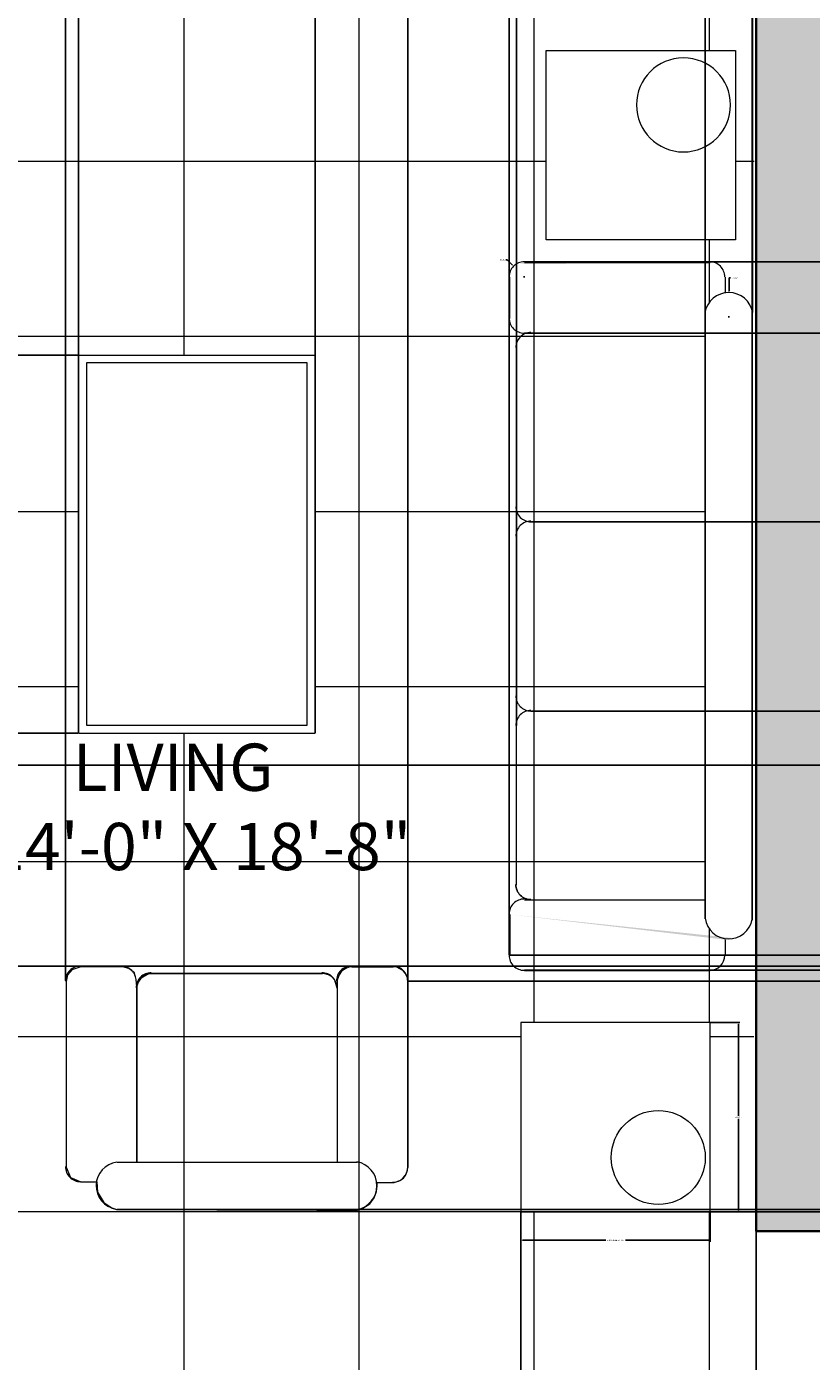
# Model space of a CAD drawing. Units: inches. Extents: x 6 to 575, y 34 to 566.
# Tile 15 of 21: x 282 to 382, y 262 to 432. Entities that reach past the tile are written whole.
import ezdxf

# ---------------------------------------------------------------- set-up
doc = ezdxf.new("R2010")
doc.units = ezdxf.units.IN
doc.linetypes.add('ACAD_ISO02W100', pattern=[15, 12, -3])
for name, color, linetype, lineweight in [('A-ANNO-DIMS', 2, 'Continuous', 18), ('A-AREA-IDEN', 6, 'Continuous', 20), ('A-FLOR-PATT', 252, 'Continuous', 9), ('A-WALL-OVHD', 7, 'ACAD_ISO02W100', 18), ('A-WALL-PATT', 251, 'Continuous', 9), ('FUR', 2, 'Continuous', 18), ('WALLS', 7, 'Continuous', 35)]:
    doc.layers.add(name, color=color, linetype=linetype, lineweight=lineweight)
doc.styles.add('PDF Arial Narrow', font='txt')
doc.styles.get("Standard").update_dxf_attribs({"font": 'arial.ttf'})
doc.dimstyles.get("Standard").update_dxf_attribs({"dimtxt": 0.18, "dimasz": 0.18, "dimexe": 0.18, "dimexo": 0.0625, "dimgap": 0.09, "dimtad": 0, "dimtih": 1, "dimtoh": 1, "dimdec": 4, "dimzin": 0, "dimdsep": 46, "dimtxsty": 'Standard', "dimcen": 0.09, "dimadec": 0, "dimazin": 0, "dimtfac": 1, "dimtdec": 4, "dimtofl": 0, "dimtmove": 0, "dimatfit": 3, "dimfxl": 1, "dimtolj": 1, "dimtzin": 0, "dimarcsym": 0})

# ---------------------------------------------------------------- blocks, each defined once
blk = doc.blocks.new('TABLE-END-24IN')
blk.add_lwpolyline([(24.03, 24.03), (0, 24.03), (0, 0), (24.03, 0)], close=True)
blk.add_circle((17.44, 6.9), 5.97)
blk = doc.blocks.new('*D27')
at = {"layer": 'A-ANNO-DIMS', "color": 0, "lineweight": -2, "transparency": 16777216}
for p, q in [((344.78, 281.17), (344.78, 277.45)), ((368.81, 281.17), (368.81, 277.45)), ((344.96, 277.63), (355.54, 277.63)), ((368.63, 277.63), (358.05, 277.63))]:
    blk.add_line(p, q, dxfattribs=at)
at = {"layer": 'A-ANNO-DIMS', "color": 0, "transparency": 16777216}
for points in [[(344.96, 277.66), (344.96, 277.6), (344.78, 277.63)], [(368.63, 277.66), (368.63, 277.6), (368.81, 277.63)]]:
    blk.add_solid(points, dxfattribs=at)
at = {"layer": 'Defpoints', "color": 0, "transparency": 16777216}
for p in [(344.78, 281.24), (368.81, 281.24), (368.81, 277.63)]:
    blk.add_point(p, dxfattribs=at)
at = {"layer": 'A-ANNO-DIMS', "color": 0, "transparency": 16777216, "insert": (356.79, 277.63), "char_height": 0.18, "attachment_point": 5}
blk.add_mtext('\\A1;END TABLE 24 TYP.', dxfattribs=at)
blk = doc.blocks.new('*D28')
at = {"layer": 'A-ANNO-DIMS', "color": 0, "lineweight": -2, "transparency": 16777216}
for p, q in [((368.87, 305.27), (372.59, 305.27)), ((372.41, 305.09), (372.41, 293.43)), ((372.41, 281.42), (372.41, 293.07)), ((368.87, 281.24), (372.59, 281.24))]:
    blk.add_line(p, q, dxfattribs=at)
at = {"layer": 'A-ANNO-DIMS', "color": 0, "transparency": 16777216}
for points in [[(372.38, 305.09), (372.44, 305.09), (372.41, 305.27)], [(372.38, 281.42), (372.44, 281.42), (372.41, 281.24)]]:
    blk.add_solid(points, dxfattribs=at)
at = {"layer": 'Defpoints', "color": 0, "transparency": 16777216}
for p in [(368.81, 305.27), (372.41, 305.27), (368.81, 281.24)]:
    blk.add_point(p, dxfattribs=at)
at = {"layer": 'A-ANNO-DIMS', "color": 0, "transparency": 16777216, "insert": (372.41, 293.25), "char_height": 0.18, "attachment_point": 5}
blk.add_mtext('\\A1;24 TYP.', dxfattribs=at)
blk = doc.blocks.new('*D54')
at = {"layer": 'A-ANNO-DIMS', "color": 0, "lineweight": -2, "transparency": 16777216}
for p, q in [((444.96, 337.94), (6.65, 337.94)), ((6.83, 337.76), (6.83, 299.11)), ((6.83, 260.1), (6.83, 298.75)), ((444.96, 259.92), (6.65, 259.92))]:
    blk.add_line(p, q, dxfattribs=at)
at = {"layer": 'A-ANNO-DIMS', "color": 0, "transparency": 16777216}
for points in [[(6.8, 337.76), (6.86, 337.76), (6.83, 337.94)], [(6.8, 260.1), (6.86, 260.1), (6.83, 259.92)]]:
    blk.add_solid(points, dxfattribs=at)
at = {"layer": 'Defpoints', "color": 0, "transparency": 16777216}
for p in [(6.83, 337.94), (445.02, 337.94), (445.02, 259.92)]:
    blk.add_point(p, dxfattribs=at)
at = {"layer": 'A-ANNO-DIMS', "color": 0, "transparency": 16777216, "insert": (6.83, 298.93), "char_height": 0.18, "attachment_point": 5}
blk.add_mtext('\\A1;78.02', dxfattribs=at)
blk = doc.blocks.new('*D119')
at = {"layer": 'A-ANNO-DIMS', "color": 0, "lineweight": -2, "transparency": 16777216}
for p, q in [((343.28, 400.02), (343.28, 565.81)), ((343.46, 565.63), (358.36, 565.63)), ((374.01, 565.63), (359.11, 565.63)), ((374.19, 395.44), (374.19, 565.81))]:
    blk.add_line(p, q, dxfattribs=at)
at = {"layer": 'A-ANNO-DIMS', "color": 0, "transparency": 16777216}
for points in [[(343.46, 565.66), (343.46, 565.6), (343.28, 565.63)], [(374.01, 565.66), (374.01, 565.6), (374.19, 565.63)]]:
    blk.add_solid(points, dxfattribs=at)
at = {"layer": 'Defpoints', "color": 0, "transparency": 16777216}
for p in [(374.19, 565.63), (343.28, 399.96), (374.19, 395.38)]:
    blk.add_point(p, dxfattribs=at)
at = {"layer": 'A-ANNO-DIMS', "color": 0, "transparency": 16777216, "insert": (358.73, 565.63), "char_height": 0.18, "attachment_point": 5}
blk.add_mtext('\\A1;30.91', dxfattribs=at)
blk = doc.blocks.new('*D120')
at = {"layer": 'A-ANNO-DIMS', "color": 0, "lineweight": -2, "transparency": 16777216}
for p, q in [((345.25, 401.87), (574.68, 401.87)), ((574.5, 401.69), (574.5, 357.07)), ((574.5, 312.09), (574.5, 356.71)), ((345.25, 311.91), (574.68, 311.91))]:
    blk.add_line(p, q, dxfattribs=at)
at = {"layer": 'A-ANNO-DIMS', "color": 0, "transparency": 16777216}
for points in [[(574.47, 401.69), (574.53, 401.69), (574.5, 401.87)], [(574.47, 312.09), (574.53, 312.09), (574.5, 311.91)]]:
    blk.add_solid(points, dxfattribs=at)
at = {"layer": 'Defpoints', "color": 0, "transparency": 16777216}
for p in [(345.19, 401.87), (574.5, 401.87), (345.19, 311.91)]:
    blk.add_point(p, dxfattribs=at)
at = {"layer": 'A-ANNO-DIMS', "color": 0, "transparency": 16777216, "insert": (574.5, 356.89), "char_height": 0.18, "attachment_point": 5}
blk.add_mtext('\\A1;89.96', dxfattribs=at)
blk = doc.blocks.new('*D121')
at = {"layer": 'A-ANNO-DIMS', "color": 0, "lineweight": -2, "transparency": 16777216}
for p, q in [((345.25, 311.91), (574.68, 311.91)), ((574.5, 311.73), (574.5, 296.75)), ((574.5, 281.42), (574.5, 296.39)), ((344.84, 281.24), (574.68, 281.24))]:
    blk.add_line(p, q, dxfattribs=at)
at = {"layer": 'A-ANNO-DIMS', "color": 0, "transparency": 16777216}
for points in [[(574.47, 311.73), (574.53, 311.73), (574.5, 311.91)], [(574.47, 281.42), (574.53, 281.42), (574.5, 281.24)]]:
    blk.add_solid(points, dxfattribs=at)
at = {"layer": 'Defpoints', "color": 0, "transparency": 16777216}
for p in [(345.19, 311.91), (574.5, 311.91), (344.78, 281.24)]:
    blk.add_point(p, dxfattribs=at)
at = {"layer": 'A-ANNO-DIMS', "color": 0, "transparency": 16777216, "insert": (574.5, 296.57), "char_height": 0.18, "attachment_point": 5}
blk.add_mtext('\\A1;30.673', dxfattribs=at)
blk = doc.blocks.new('*D122')
at = {"layer": 'A-ANNO-DIMS', "color": 0, "lineweight": -2, "transparency": 16777216}
for p, q in [((344.78, 281.17), (344.78, 33.76)), ((374.66, 278.74), (374.66, 33.76)), ((344.96, 33.94), (359.32, 33.94)), ((374.48, 33.94), (360.11, 33.94))]:
    blk.add_line(p, q, dxfattribs=at)
at = {"layer": 'A-ANNO-DIMS', "color": 0, "transparency": 16777216}
for points in [[(344.96, 33.97), (344.96, 33.91), (344.78, 33.94)], [(374.48, 33.97), (374.48, 33.91), (374.66, 33.94)]]:
    blk.add_solid(points, dxfattribs=at)
at = {"layer": 'Defpoints', "color": 0, "transparency": 16777216}
for p in [(344.78, 281.24), (374.66, 278.8), (344.78, 33.94)]:
    blk.add_point(p, dxfattribs=at)
at = {"layer": 'A-ANNO-DIMS', "color": 0, "transparency": 16777216, "insert": (359.72, 33.94), "char_height": 0.18, "attachment_point": 5}
blk.add_mtext('\\A1;29.88', dxfattribs=at)
blk = doc.blocks.new('*D123')
at = {"layer": 'A-ANNO-DIMS', "color": 0, "lineweight": -2, "transparency": 16777216}
for p, q in [((344.84, 281.24), (574.68, 281.24)), ((574.5, 281.06), (574.5, 280.2)), ((574.5, 278.98), (574.5, 279.84)), ((374.72, 278.8), (574.68, 278.8))]:
    blk.add_line(p, q, dxfattribs=at)
at = {"layer": 'A-ANNO-DIMS', "color": 0, "transparency": 16777216}
for points in [[(574.47, 281.06), (574.53, 281.06), (574.5, 281.24)], [(574.47, 278.98), (574.53, 278.98), (574.5, 278.8)]]:
    blk.add_solid(points, dxfattribs=at)
at = {"layer": 'Defpoints', "color": 0, "transparency": 16777216}
for p in [(344.78, 281.24), (574.5, 281.24), (374.66, 278.8)]:
    blk.add_point(p, dxfattribs=at)
at = {"layer": 'A-ANNO-DIMS', "color": 0, "transparency": 16777216, "insert": (574.5, 280.02), "char_height": 0.18, "attachment_point": 5}
blk.add_mtext('\\A1;2.435', dxfattribs=at)
blk = doc.blocks.new('*D124')
at = {"layer": 'A-ANNO-DIMS', "color": 0, "lineweight": -2, "transparency": 16777216}
for p, q in [((345.25, 401.87), (574.68, 401.87)), ((574.5, 401.69), (574.5, 397.53)), ((574.5, 393), (574.5, 397.16)), ((345.25, 392.82), (574.68, 392.82))]:
    blk.add_line(p, q, dxfattribs=at)
at = {"layer": 'A-ANNO-DIMS', "color": 0, "transparency": 16777216}
for points in [[(574.47, 401.69), (574.53, 401.69), (574.5, 401.87)], [(574.47, 393), (574.53, 393), (574.5, 392.82)]]:
    blk.add_solid(points, dxfattribs=at)
at = {"layer": 'Defpoints', "color": 0, "transparency": 16777216}
for p in [(345.19, 401.87), (574.5, 401.87), (345.19, 392.82)]:
    blk.add_point(p, dxfattribs=at)
at = {"layer": 'A-ANNO-DIMS', "color": 0, "transparency": 16777216, "insert": (574.5, 397.34), "char_height": 0.18, "attachment_point": 5}
blk.add_mtext('\\A1;9.05', dxfattribs=at)
blk = doc.blocks.new('*D125')
at = {"layer": 'A-ANNO-DIMS', "color": 0, "lineweight": -2, "transparency": 16777216}
for p, q in [((346.11, 368.87), (574.68, 368.87)), ((574.5, 368.69), (574.5, 357.03)), ((574.5, 345.01), (574.5, 356.67)), ((346.11, 344.83), (574.68, 344.83))]:
    blk.add_line(p, q, dxfattribs=at)
at = {"layer": 'A-ANNO-DIMS', "color": 0, "transparency": 16777216}
for points in [[(574.47, 368.69), (574.53, 368.69), (574.5, 368.87)], [(574.47, 345.01), (574.53, 345.01), (574.5, 344.83)]]:
    blk.add_solid(points, dxfattribs=at)
at = {"layer": 'Defpoints', "color": 0, "transparency": 16777216}
for p in [(346.05, 368.87), (574.5, 368.87), (346.05, 344.83)]:
    blk.add_point(p, dxfattribs=at)
at = {"layer": 'A-ANNO-DIMS', "color": 0, "transparency": 16777216, "insert": (574.5, 356.85), "char_height": 0.18, "attachment_point": 5}
blk.add_mtext('\\A1;24.03', dxfattribs=at)
blk = doc.blocks.new('*D126')
at = {"layer": 'A-ANNO-DIMS', "color": 0, "lineweight": -2, "transparency": 16777216}
for p, q in [((368.18, 318.51), (368.18, 565.81)), ((368.36, 565.63), (370.78, 565.63)), ((373.95, 565.63), (371.53, 565.63)), ((374.13, 318.46), (374.13, 565.81))]:
    blk.add_line(p, q, dxfattribs=at)
at = {"layer": 'A-ANNO-DIMS', "color": 0, "transparency": 16777216}
for points in [[(368.36, 565.66), (368.36, 565.6), (368.18, 565.63)], [(373.95, 565.66), (373.95, 565.6), (374.13, 565.63)]]:
    blk.add_solid(points, dxfattribs=at)
at = {"layer": 'Defpoints', "color": 0, "transparency": 16777216}
for p in [(374.13, 565.63), (368.18, 318.45), (374.13, 318.4)]:
    blk.add_point(p, dxfattribs=at)
at = {"layer": 'A-ANNO-DIMS', "color": 0, "transparency": 16777216, "insert": (371.16, 565.63), "char_height": 0.18, "attachment_point": 5}
blk.add_mtext('\\A1;5.951', dxfattribs=at)
blk = doc.blocks.new('*D127')
at = {"layer": 'A-ANNO-DIMS', "color": 0, "lineweight": -2, "transparency": 16777216}
for p, q in [((286.95, 310.61), (286.95, 565.81)), ((287.13, 565.63), (308.28, 565.63)), ((330.22, 565.63), (309.07, 565.63)), ((330.4, 310.61), (330.4, 565.81))]:
    blk.add_line(p, q, dxfattribs=at)
at = {"layer": 'A-ANNO-DIMS', "color": 0, "transparency": 16777216}
for points in [[(287.13, 565.66), (287.13, 565.6), (286.95, 565.63)], [(330.22, 565.66), (330.22, 565.6), (330.4, 565.63)]]:
    blk.add_solid(points, dxfattribs=at)
at = {"layer": 'Defpoints', "color": 0, "transparency": 16777216}
for p in [(330.4, 565.63), (286.95, 310.54), (330.4, 310.54)]:
    blk.add_point(p, dxfattribs=at)
at = {"layer": 'A-ANNO-DIMS', "color": 0, "transparency": 16777216, "insert": (308.68, 565.63), "char_height": 0.18, "attachment_point": 5}
blk.add_mtext('\\A1;43.46', dxfattribs=at)
blk = doc.blocks.new('*D128')
at = {"layer": 'A-ANNO-DIMS', "color": 0, "lineweight": -2, "transparency": 16777216}
for p, q in [((288.92, 312.45), (574.68, 312.45)), ((574.5, 312.27), (574.5, 297.18)), ((574.5, 281.73), (574.5, 296.82)), ((293.5, 281.55), (574.68, 281.55))]:
    blk.add_line(p, q, dxfattribs=at)
at = {"layer": 'A-ANNO-DIMS', "color": 0, "transparency": 16777216}
for points in [[(574.47, 312.27), (574.53, 312.27), (574.5, 312.45)], [(574.47, 281.73), (574.53, 281.73), (574.5, 281.55)]]:
    blk.add_solid(points, dxfattribs=at)
at = {"layer": 'Defpoints', "color": 0, "transparency": 16777216}
for p in [(288.86, 312.45), (574.5, 312.45), (293.44, 281.55)]:
    blk.add_point(p, dxfattribs=at)
at = {"layer": 'A-ANNO-DIMS', "color": 0, "transparency": 16777216, "insert": (574.5, 297), "char_height": 0.18, "attachment_point": 5}
blk.add_mtext('\\A1;30.91', dxfattribs=at)
blk = doc.blocks.new('*D129')
at = {"layer": 'A-ANNO-DIMS', "color": 0, "lineweight": -2, "transparency": 16777216}
for p, q in [((330.4, 310.61), (330.4, 565.81)), ((330.58, 565.63), (336.39, 565.63)), ((343.1, 565.63), (337.3, 565.63)), ((343.28, 313.88), (343.28, 565.81))]:
    blk.add_line(p, q, dxfattribs=at)
at = {"layer": 'A-ANNO-DIMS', "color": 0, "transparency": 16777216}
for points in [[(330.58, 565.66), (330.58, 565.6), (330.4, 565.63)], [(343.1, 565.66), (343.1, 565.6), (343.28, 565.63)]]:
    blk.add_solid(points, dxfattribs=at)
at = {"layer": 'Defpoints', "color": 0, "transparency": 16777216}
for p in [(343.28, 565.63), (343.28, 313.82), (330.4, 310.54)]:
    blk.add_point(p, dxfattribs=at)
at = {"layer": 'A-ANNO-DIMS', "color": 0, "transparency": 16777216, "insert": (336.84, 565.63), "char_height": 0.18, "attachment_point": 5}
blk.add_mtext('\\A1;12.874', dxfattribs=at)
blk = doc.blocks.new('*D130')
at = {"layer": 'A-ANNO-DIMS', "color": 0, "lineweight": -2, "transparency": 16777216}
for p, q in [((343.34, 313.82), (574.68, 313.82)), ((574.5, 313.64), (574.5, 312.36)), ((574.5, 310.72), (574.5, 312)), ((330.47, 310.54), (574.68, 310.54))]:
    blk.add_line(p, q, dxfattribs=at)
at = {"layer": 'A-ANNO-DIMS', "color": 0, "transparency": 16777216}
for points in [[(574.47, 313.64), (574.53, 313.64), (574.5, 313.82)], [(574.47, 310.72), (574.53, 310.72), (574.5, 310.54)]]:
    blk.add_solid(points, dxfattribs=at)
at = {"layer": 'Defpoints', "color": 0, "transparency": 16777216}
for p in [(343.28, 313.82), (574.5, 313.82), (330.4, 310.54)]:
    blk.add_point(p, dxfattribs=at)
at = {"layer": 'A-ANNO-DIMS', "color": 0, "transparency": 16777216, "insert": (574.5, 312.18), "char_height": 0.18, "attachment_point": 5}
blk.add_mtext('\\A1;3.277', dxfattribs=at)
blk = doc.blocks.new('*D131')
at = {"layer": 'A-ANNO-DIMS', "color": 0, "lineweight": -2, "transparency": 16777216}
for p, q in [((288.6, 342.08), (288.6, 565.81)), ((288.78, 565.63), (303.23, 565.63)), ((318.46, 565.63), (304.02, 565.63)), ((318.64, 342.08), (318.64, 565.81))]:
    blk.add_line(p, q, dxfattribs=at)
at = {"layer": 'A-ANNO-DIMS', "color": 0, "transparency": 16777216}
for points in [[(288.78, 565.66), (288.78, 565.6), (288.6, 565.63)], [(318.46, 565.66), (318.46, 565.6), (318.64, 565.63)]]:
    blk.add_solid(points, dxfattribs=at)
at = {"layer": 'Defpoints', "color": 0, "transparency": 16777216}
for p in [(318.64, 565.63), (288.6, 342.01), (318.64, 342.01)]:
    blk.add_point(p, dxfattribs=at)
at = {"layer": 'A-ANNO-DIMS', "color": 0, "transparency": 16777216, "insert": (303.62, 565.63), "char_height": 0.18, "attachment_point": 5}
blk.add_mtext('\\A1;30.04', dxfattribs=at)
blk = doc.blocks.new('*D132')
at = {"layer": 'A-ANNO-DIMS', "color": 0, "lineweight": -2, "transparency": 16777216}
for p, q in [((288.54, 390), (6.65, 390)), ((6.83, 389.82), (6.83, 366.19)), ((6.83, 342.19), (6.83, 365.82)), ((288.54, 342.01), (6.65, 342.01))]:
    blk.add_line(p, q, dxfattribs=at)
at = {"layer": 'A-ANNO-DIMS', "color": 0, "transparency": 16777216}
for points in [[(6.8, 389.82), (6.86, 389.82), (6.83, 390)], [(6.8, 342.19), (6.86, 342.19), (6.83, 342.01)]]:
    blk.add_solid(points, dxfattribs=at)
at = {"layer": 'Defpoints', "color": 0, "transparency": 16777216}
for p in [(6.83, 390), (288.6, 390), (288.6, 342.01)]:
    blk.add_point(p, dxfattribs=at)
at = {"layer": 'A-ANNO-DIMS', "color": 0, "transparency": 16777216, "insert": (6.83, 366), "char_height": 0.18, "attachment_point": 5}
blk.add_mtext('\\A1;47.98', dxfattribs=at)
blk = doc.blocks.new('*D133')
at = {"layer": 'A-ANNO-DIMS', "color": 0, "lineweight": -2, "transparency": 16777216}
for p, q in [((288.54, 342.01), (6.65, 342.01)), ((6.83, 341.83), (6.83, 327.42)), ((6.83, 312.63), (6.83, 327.05)), ((288.79, 312.45), (6.65, 312.45))]:
    blk.add_line(p, q, dxfattribs=at)
at = {"layer": 'A-ANNO-DIMS', "color": 0, "transparency": 16777216}
for points in [[(6.8, 341.83), (6.86, 341.83), (6.83, 342.01)], [(6.8, 312.63), (6.86, 312.63), (6.83, 312.45)]]:
    blk.add_solid(points, dxfattribs=at)
at = {"layer": 'Defpoints', "color": 0, "transparency": 16777216}
for p in [(288.6, 342.01), (6.83, 312.45), (288.86, 312.45)]:
    blk.add_point(p, dxfattribs=at)
at = {"layer": 'A-ANNO-DIMS', "color": 0, "transparency": 16777216, "insert": (6.83, 327.23), "char_height": 0.18, "attachment_point": 5}
blk.add_mtext('\\A1;29.56', dxfattribs=at)
blk = doc.blocks.new('*D134')
at = {"layer": 'A-ANNO-DIMS', "color": 0, "lineweight": -2, "transparency": 16777216}
for p, q in [((318.64, 342.08), (318.64, 565.81)), ((318.82, 565.63), (331.04, 565.63)), ((344.05, 565.63), (331.83, 565.63)), ((344.23, 343.01), (344.23, 565.81))]:
    blk.add_line(p, q, dxfattribs=at)
at = {"layer": 'A-ANNO-DIMS', "color": 0, "transparency": 16777216}
for points in [[(318.82, 565.66), (318.82, 565.6), (318.64, 565.63)], [(344.05, 565.66), (344.05, 565.6), (344.23, 565.63)]]:
    blk.add_solid(points, dxfattribs=at)
at = {"layer": 'Defpoints', "color": 0, "transparency": 16777216}
for p in [(344.23, 565.63), (344.23, 342.95), (318.64, 342.01)]:
    blk.add_point(p, dxfattribs=at)
at = {"layer": 'A-ANNO-DIMS', "color": 0, "transparency": 16777216, "insert": (331.44, 565.63), "char_height": 0.18, "attachment_point": 5}
blk.add_mtext('\\A1;25.59', dxfattribs=at)
blk = doc.blocks.new('*D244')
at = {"layer": 'A-ANNO-DIMS', "color": 0, "lineweight": -2, "transparency": 16777216}
for p, q in [((342.85, 402.12), (343.03, 402.12)), ((343.03, 402.12), (343.71, 401.44)), ((345.1, 399.96), (345.28, 399.96)), ((345.19, 399.87), (345.19, 400.05))]:
    blk.add_line(p, q, dxfattribs=at)
at = {"layer": 'A-ANNO-DIMS', "color": 0, "transparency": 16777216}
blk.add_solid([(343.73, 401.46), (343.69, 401.42), (343.84, 401.31)], dxfattribs=at)
at = {"layer": 'Defpoints', "color": 0, "transparency": 16777216}
for p in [(343.84, 401.31), (345.19, 399.96)]:
    blk.add_point(p, dxfattribs=at)
at = {"layer": 'A-ANNO-DIMS', "color": 0, "transparency": 16777216, "insert": (342.46, 402.12), "char_height": 0.18, "attachment_point": 5}
blk.add_mtext('\\A1;R1.91', dxfattribs=at)
blk = doc.blocks.new('*D245')
at = {"layer": 'A-ANNO-DIMS', "color": 0, "lineweight": -2, "transparency": 16777216}
for p, q in [((371.22, 399.82), (371.2, 398.15)), ((371.4, 399.82), (371.22, 399.82)), ((371.08, 394.89), (371.26, 394.89)), ((371.17, 394.8), (371.17, 394.98))]:
    blk.add_line(p, q, dxfattribs=at)
at = {"layer": 'A-ANNO-DIMS', "color": 0, "transparency": 16777216}
blk.add_solid([(371.17, 398.15), (371.23, 398.15), (371.2, 397.97)], dxfattribs=at)
at = {"layer": 'Defpoints', "color": 0, "transparency": 16777216}
for p in [(371.2, 397.97), (371.17, 394.89)]:
    blk.add_point(p, dxfattribs=at)
at = {"layer": 'A-ANNO-DIMS', "color": 0, "transparency": 16777216, "insert": (371.88, 399.82), "char_height": 0.18, "attachment_point": 5}
blk.add_mtext('\\A1;R3.082', dxfattribs=at)

msp = doc.modelspace()

# ---------------------------------------------------------------- hatches: boundary and pattern name
at = {"layer": 'A-FLOR-PATT'}
h = msp.add_hatch(dxfattribs=at)
h.set_pattern_fill('NET', color=256, scale=7)
h.set_pattern_definition([(0, (-98.035, 170.147), (0, 22.225), []), (90, (-98.035, 170.147), (-22.225, 1e-15), [])])
h.paths.add_polyline_path([(368.183, 395.6385, -0.88370529), (374.2533, 394.8861), (374.6586, 448.801), (354.6586, 448.801), (354.6586, 448.7938), (353.1847, 448.7938), (326.6586, 448.801), (322.6586, 448.801), (248.6332, 448.8024), (206.6586, 448.8024), (206.6586, 389.449), (221.6622, 389.449), (221.6622, 310.5712), (206.6586, 310.5712), (206.6586, 276.801), (206.6704, 276.801), (206.6704, 274.3795), (206.6586, 224.801), (246.6586, 224.801), (264.6586, 224.801), (265.6986, 224.801), (265.6986, 249.081), (267.5186, 249.081), (267.5186, 249.0145, -0.38515288), (290.6494, 224.801), (290.6679, 224.801, -0.38515288), (313.7986, 249.0145), (313.7986, 249.081), (315.6186, 249.081), (315.6186, 224.801), (316.6586, 224.801), (334.6586, 224.801), (374.6586, 224.801), (374.6586, 278.801), (374.1753, 318.8919, -0.45530286), (370.7577, 315.9168), (370.6643, 313.8205, -0.41421356), (368.7528, 311.909), (368.8072, 311.8975), (368.7528, 311.909, 0.41421356), (370.6643, 313.8205), (370.7632, 315.9161, -0.34634601), (368.183, 318.5897)])
h.paths.add_polyline_path([(288.603, 342.0131), (288.603, 389.9952), (318.6406, 389.9952), (318.6406, 342.0131)], flags=16)
h.paths.add_polyline_path([(289.6173, 343.0274), (289.6173, 389.059), (317.6263, 389.059), (317.6263, 343.0274)], flags=0)
h.paths.add_polyline_path([(295.4867, 311.7535, 0.06538163), (295.1241, 312.0945), (295.0006, 312.1316)], flags=16)
h.paths.add_polyline_path([(328.4931, 284.9911, 0.41421356), (330.4045, 286.9026), (330.4215, 286.8532), (330.4045, 286.9026, -0.41421356), (328.4931, 284.9911), (328.549, 284.9808)], flags=16)
h.paths.add_polyline_path([(344.7771, 305.2659), (368.8072, 305.2659), (368.8072, 281.2358), (344.7771, 281.2358)], flags=16)
h.paths.add_polyline_path([(368.183, 288.1406, -1), (356.246, 288.1406, -1)], flags=0)
h.paths.add_polyline_path([(347.9759, 404.6629), (347.9759, 428.6929), (372.006, 428.6929), (372.006, 404.6629)], flags=16)
h.paths.add_polyline_path([(359.4448, 421.7882, -1), (371.3818, 421.7882, -1)], flags=0)
at = {"layer": 'A-WALL-PATT'}
h = msp.add_hatch(color=256, dxfattribs=at)
h.dxf.hatch_style = 1
h.paths.add_polyline_path([(160.6586, 539.801), (32.6586, 539.801), (32.6586, 272.801), (41.6586, 272.801), (41.6586, 286.0643), (41.6586, 358.0764), (41.6586, 379.0637), (41.6586, 407.7709), (41.6194, 407.7709), (41.6194, 431.801), (82.8918, 431.801), (82.8918, 440.801), (65.6494, 440.801), (65.6494, 440.7732), (41.6194, 440.7732), (41.6194, 515.5941), (41.6586, 530.801), (117.6586, 530.801), (117.6586, 474.801), (120.6068, 474.801), (121.6586, 474.801), (121.6586, 530.801), (137.4275, 530.801), (137.4275, 530.8356), (141.2505, 530.8356), (160.6586, 530.801)])
h.paths.add_polyline_path([(71.6586, 212.801), (41.6586, 212.801), (41.6586, 224.801), (32.6586, 224.801), (32.6586, 203.801), (71.6586, 203.801)])
h.paths.add_polyline_path([(206.6586, 215.801), (246.6586, 215.801), (246.6586, 224.801), (206.6586, 224.801), (206.6586, 230.801), (201.8157, 230.801), (197.6586, 230.801), (197.6586, 212.801), (167.6586, 212.801), (167.6586, 203.801), (206.6586, 203.801)])
h.paths.add_polyline_path([(383.6586, 224.801), (334.6586, 224.801), (334.6586, 215.801), (374.6586, 215.801), (374.6586, 203.801), (384.0753, 203.801), (407.6586, 203.801), (407.6586, 212.801), (383.6586, 212.801)])
h.paths.add_polyline_path([(548.6586, 270.801), (539.6586, 270.801), (539.6586, 212.801), (515.6586, 212.801), (515.6586, 203.801), (548.6586, 203.801)])
h.paths.add_polyline_path([(548.6586, 412.801), (545.7108, 412.801), (539.6586, 412.801), (539.6586, 382.801), (433.708, 382.801), (433.708, 378.801), (539.6586, 378.801), (539.6586, 366.801), (548.6586, 366.801)])
h.paths.add_polyline_path([(548.6586, 539.801), (455.9436, 539.801), (455.9436, 530.801), (539.6586, 530.801), (539.6586, 440.801), (548.6586, 440.801)])
h.paths.add_polyline_path([(407.9436, 539.801), (362.6586, 539.801), (362.6586, 530.801), (374.6586, 530.801), (374.6586, 452.801), (354.6586, 452.801), (354.6586, 448.801), (374.6586, 448.801), (374.6586, 278.801), (383.6586, 278.801), (383.6586, 530.801), (407.9436, 530.801)])
h.paths.add_polyline_path([(338.6586, 539.801), (320.6586, 539.801), (320.6586, 530.801), (322.6586, 530.801), (322.6586, 448.801), (326.6586, 448.801), (326.6586, 530.801), (338.6586, 530.801)])
h.paths.add_polyline_path([(272.6586, 539.801), (184.6586, 539.801), (184.6586, 530.801), (197.6586, 530.801), (197.6586, 440.801), (176.6714, 440.801), (121.6586, 440.801), (121.6586, 446.801), (117.6586, 446.801), (117.6586, 440.801), (111.6586, 440.801), (111.6586, 431.801), (197.6586, 431.801), (197.6586, 407.7709), (197.6586, 276.801), (206.6586, 276.801), (206.6586, 530.801), (272.6586, 530.801)])

# ---------------------------------------------------------------- linework, layer by layer
at = {"layer": 'A-WALL-OVHD', "ltscale": 0.3}
msp.add_line((374.6586, 278.801), (374.6586, 224.801), dxfattribs=at)
at = {"layer": 'FUR'}
for p, q in [((346.0482, 368.8656), (368.183, 368.8656)), ((346.0482, 344.8346), (368.183, 344.8346))]:
    msp.add_line(p, q, dxfattribs=at)
for points in [[(347.9759, 404.6629), (347.9759, 428.6929), (372.006, 428.6929), (372.006, 404.6629)], [(288.603, 389.9952), (288.603, 342.0131), (318.6406, 342.0131), (318.6406, 389.9952)], [(289.6173, 389.059), (289.6173, 343.0274), (317.6263, 343.0274), (317.6263, 389.059)], [(330.4215, 288.3356), (330.4215, 310.0251), (330.4215, 310.4932), (330.4215, 310.8833), (330.2655, 311.1954), (330.1094, 311.5074), (329.8754, 311.8195), (329.6413, 311.9756), (329.3292, 312.1316), (329.0172, 312.2876), (328.7051, 312.3657), (323.7898, 312.3657), (322.9316, 312.2876), (322.5415, 312.1316), (321.9954, 311.8195), (321.6833, 311.3514), (321.4493, 310.6492), (321.4493, 310.0251), (321.4493, 309.635), (321.1372, 310.6492), (320.7471, 311.1173), (320.357, 311.3514), (319.7328, 311.5074), (299.1356, 311.5074), (297.4192, 311.4294), (297.0291, 311.2734), (296.483, 310.9613), (296.2489, 310.5712), (296.0149, 310.1031), (296.0149, 309.713), (296.0149, 309.869), (296.3269, 310.6492), (296.561, 310.9613), (297.4972, 311.5074), (300.2279, 311.5074), (297.8873, 311.5074), (296.9511, 311.2734), (296.561, 310.9613), (296.0929, 310.2591), (296.0149, 309.869), (295.9368, 310.7272), (295.7028, 311.5855), (295.0006, 312.1316), (294.2204, 312.3657), (293.2062, 312.3657), (288.9151, 312.3657), (287.7448, 311.9756), (287.1986, 311.3514), (287.0426, 310.4932), (287.0426, 286.9313), (287.5887, 285.6049), (288.9151, 285.0588), (290.3194, 285.0588), (290.9436, 285.0588), (291.0216, 283.7325), (291.8018, 282.4061), (292.8941, 281.7039), (293.4402, 281.5479), (318.8746, 281.4699), (324.0239, 281.4699), (324.7261, 281.7039), (325.5843, 282.2501), (326.1304, 283.0303), (326.4425, 283.8105), (326.5205, 284.5127), (326.5205, 284.9808), (327.7689, 284.9808), (328.7051, 284.9808), (329.4073, 285.2148), (329.8754, 285.5269), (330.1094, 285.839), (330.3435, 286.3851), (330.4215, 286.8532), (330.4215, 289.0378)]]:
    msp.add_lwpolyline(points, close=True, dxfattribs=at)
for points in [[(345.2452, 401.7761), (368.8072, 401.7761)], [(343.3728, 394.6764), (343.3728, 399.9037)], [(370.7577, 397.8752), (370.7577, 399.9037)], [(368.183, 318.4512), (368.183, 395.3785)], [(374.1905, 318.2952), (374.1905, 395.3785)], [(345.2452, 392.8039), (368.183, 392.8039)], [(344.231, 370.7243), (344.231, 390.9314)], [(344.231, 346.6943), (344.231, 366.9794)], [(344.231, 322.7423), (344.231, 342.9494)], [(345.2452, 320.8698), (368.183, 320.8698)], [(343.3728, 318.9973), (343.3728, 313.77)], [(370.7577, 313.77), (370.7577, 315.7985)], [(294.1424, 312.3657), (288.9151, 312.3657)], [(323.3217, 312.3657), (328.549, 312.3657)], [(345.2452, 311.8975), (368.8072, 311.8975)], [(287.0426, 310.4932), (287.0426, 286.9313)], [(296.0149, 309.635), (296.0149, 287.5554), (296.0149, 310.4932)], [(297.8873, 311.5074), (319.5768, 311.5074)], [(321.4493, 310.4932), (321.4493, 287.5554)], [(330.4215, 310.4932), (330.4215, 286.8532)], [(296.0149, 309.713), (296.0149, 287.5554)], [(293.5182, 287.5554), (324.0239, 287.5554)], [(288.9151, 285.0588), (290.9436, 285.0588)], [(326.5205, 284.9808), (328.549, 284.9808)], [(293.4402, 281.5479), (324.0239, 281.4699)]]:
    msp.add_lwpolyline(points, dxfattribs=at)
msp.add_lwpolyline([(344.1367, 322.7931, 0.41421367), (346.0482, 320.8816, -0.41421367)], format="xyb", close=True, dxfattribs=at)
for centre, radius, start, end in [((345.1899, 399.9576), 1.9115, 89.999989, 180.000011), ((368.7528, 399.9576), 1.9115, 0, 90.000011), ((371.1715, 394.8861), 3.0818, 9.689933, 170.310067), ((345.1899, 394.7301), 1.9115, 179.999989, 270.000011), ((346.0482, 390.985), 1.9115, 89.999989, 180.000011), ((346.0482, 370.7771), 1.9115, 179.999989, 270.000011), ((346.0482, 367.032), 1.9115, 89.999989, 180.000011), ((346.0482, 346.7461), 1.9115, 179.999989, 270.000011), ((346.0482, 343.001), 1.9115, 89.999989, 180.000011), ((345.1899, 319.048), 1.9115, 89.999989, 180.000011), ((371.1715, 318.8919), 3.0038, 187.163096, 350.485836), ((345.1899, 313.8205), 1.9115, 179.999989, 270.000011), ((368.7528, 313.8205), 1.9115, 269.999989, 359.999989), ((288.8575, 310.5435), 1.9115, 89.999989, 180.000011), ((294.007, 310.5435), 1.9115, 0, 90.000011), ((323.2655, 310.5435), 1.9115, 89.999989, 180.000011), ((328.4931, 310.5435), 1.9115, 0, 90.000011), ((297.8301, 309.6853), 1.9115, 89.999989, 180.000011), ((319.5204, 309.6853), 1.9115, 0, 90.000011), ((288.8575, 286.9806), 1.9115, 179.999989, 270.000011), ((293.8509, 284.5619), 3.0038, 97.163096, 260.485836), ((323.4216, 284.5619), 3.0818, 279.689933, 80.310067), ((328.4931, 286.9026), 1.9115, 269.999989, 359.999989)]:
    msp.add_arc(centre, radius, start, end, dxfattribs=at)
at = {"layer": 'FUR', "transparency": 33554559}
for points in [[(345.2452, 401.7761), (368.8072, 401.7761), (344.4651, 401.6201)], [(370.7577, 315.7985), (343.3728, 318.9973), (372.162, 315.9546)]]:
    msp.add_solid(points, dxfattribs=at)
at = {"layer": 'WALLS'}
for q in [(374.6586, 448.801), (383.6586, 278.801)]:
    msp.add_line((374.6586, 278.801), q, dxfattribs=at)

# ---------------------------------------------------------------- block references
at = {"layer": 'FUR', "extrusion": (0, 0, -1), "zscale": -1, "rotation": 180.0000082776426}
msp.add_blockref('TABLE-END-24IN', (-347.9758, 428.6928), dxfattribs=at)
at = {"layer": 'FUR'}
msp.add_blockref('TABLE-END-24IN', (344.777, 281.236), dxfattribs=at)

# ---------------------------------------------------------------- texts
at = {"layer": 'A-AREA-IDEN', "attachment_point": 4, "style": 'PDF Arial Narrow'}
for s, insert, char_height in [('LIVING', (287.8657, 336.9155), 6.0005), ('14\'-0" X 18\'-8"', (277.2546, 326.8505), 6.000503)]:
    msp.add_mtext(s, dxfattribs=dict(at, insert=insert, char_height=char_height))

# ---------------------------------------------------------------- dimensions: what is measured, and where the dimension line sits
at = {"layer": 'A-ANNO-DIMS'}
for base, p1, p2, override, picture, middle in [((330.4045, 565.631), (286.946, 310.5435), (330.4045, 310.5435), {"dimdec": 2, "dimlfac": 1, "dimrnd": 0, "dimzin": 0, "dimdsep": 46, "dimlunit": 2}, '*D127', (308.6753, 565.631)), ((318.6406, 565.631), (288.603, 342.0131), (318.6406, 342.0131), {"dimdec": 2, "dimlfac": 1, "dimrnd": 0, "dimzin": 0, "dimdsep": 46, "dimlunit": 2}, '*D131', (303.6218, 565.631)), ((344.231, 565.631), (318.6406, 342.0131), (344.231, 342.9494), {"dimdec": 2, "dimlfac": 1, "dimrnd": 0, "dimzin": 0, "dimdsep": 46, "dimlunit": 2}, '*D134', (331.4358, 565.631)), ((343.2784, 565.631), (330.4045, 310.5435), (343.2784, 313.8205), {"dimdec": 3, "dimlfac": 1, "dimrnd": 0, "dimzin": 0, "dimdsep": 46, "dimlunit": 2}, '*D129', (336.8415, 565.631)), ((374.1905, 565.631), (343.2784, 399.9576), (374.1905, 395.3785), {"dimdec": 2, "dimlfac": 1, "dimrnd": 0, "dimzin": 0, "dimdsep": 46, "dimlunit": 2}, '*D119', (358.7345, 565.631)), ((374.134, 565.631), (368.183, 318.4512), (374.134, 318.3954), {"dimdec": 3, "dimlfac": 1, "dimrnd": 0, "dimzin": 0, "dimdsep": 46, "dimlunit": 2}, '*D126', (371.1585, 565.631)), ((344.7771, 33.9447), (374.6586, 278.801), (344.7771, 281.2358), {"dimdec": 2, "dimlfac": 1, "dimrnd": 0, "dimzin": 0, "dimdsep": 46, "dimlunit": 2}, '*D122', (359.7179, 33.9447))]:
    dim = msp.add_linear_dim(base=base, p1=p1, p2=p2, dimstyle='Standard', override=override, dxfattribs=at)
    dim.commit()
    dim.dimension.update_dxf_attribs({"geometry": picture, "text_midpoint": middle})
for center, mpoint, override, picture, middle in [((345.1899, 399.9576), (343.8395, 401.3105), {"dimdec": 2, "dimlfac": 1, "dimrnd": 0, "dimzin": 0, "dimdsep": 46, "dimlunit": 2}, '*D244', (342.4568, 402.1222)), ((371.1715, 394.8861), (371.2006, 397.9678), {"dimdec": 3, "dimlfac": 1, "dimrnd": 0, "dimzin": 0, "dimdsep": 46, "dimlunit": 2}, '*D245', (371.877, 399.8168))]:
    dim = msp.add_radius_dim(center=center, mpoint=mpoint, dimstyle='Standard', override=override, dxfattribs=at)
    dim.commit()
    dim.dimension.update_dxf_attribs({"geometry": picture, "text_midpoint": middle, "dimtype": 164})
for base, p1, p2, override, picture, middle in [((574.4958, 401.8691), (345.1899, 311.909), (345.1899, 401.8691), {"dimdec": 2, "dimlfac": 1, "dimrnd": 0, "dimzin": 0, "dimdsep": 46, "dimlunit": 2}, '*D120', (574.4958, 356.889)), ((574.4958, 401.8691), (345.1899, 392.8186), (345.1899, 401.8691), {"dimdec": 2, "dimlfac": 1, "dimrnd": 0, "dimzin": 0, "dimdsep": 46, "dimlunit": 2}, '*D124', (574.4958, 397.3439)), ((6.8286, 389.9952), (288.603, 342.0131), (288.603, 389.9952), {"dimdec": 2, "dimlfac": 1, "dimrnd": 0, "dimzin": 0, "dimdsep": 46, "dimlunit": 2}, '*D132', (6.8286, 366.0042)), ((574.4958, 368.8656), (346.0482, 344.8346), (346.0482, 368.8656), {"dimdec": 2, "dimlfac": 1, "dimrnd": 0, "dimzin": 0, "dimdsep": 46, "dimlunit": 2}, '*D125', (574.4958, 356.8501)), ((6.8286, 312.455), (288.603, 342.0131), (288.8575, 312.455), {"dimdec": 2, "dimlfac": 1, "dimrnd": 0, "dimzin": 0, "dimdsep": 46, "dimlunit": 2}, '*D133', (6.8286, 327.234)), ((6.8286, 337.9397), (445.0208, 259.9201), (445.0208, 337.9397), {"dimdec": 2, "dimlfac": 1, "dimrnd": 0, "dimzin": 0, "dimdsep": 46, "dimlunit": 2}, '*D54', (6.8286, 298.9299)), ((574.4958, 313.8205), (330.4045, 310.5435), (343.2784, 313.8205), {"dimdec": 3, "dimlfac": 1, "dimrnd": 0, "dimzin": 0, "dimdsep": 46, "dimlunit": 2}, '*D130', (574.4958, 312.182)), ((574.4958, 312.455), (293.4402, 281.5479), (288.8575, 312.455), {"dimdec": 2, "dimlfac": 1, "dimrnd": 0, "dimzin": 0, "dimdsep": 46, "dimlunit": 2}, '*D128', (574.4958, 297.0014)), ((574.4958, 311.909), (344.7771, 281.2358), (345.1899, 311.909), {"dimdec": 3, "dimlfac": 1, "dimrnd": 0, "dimzin": 0, "dimdsep": 46, "dimlunit": 2}, '*D121', (574.4958, 296.5724)), ((574.4958, 281.2358), (374.6586, 278.801), (344.7771, 281.2358), {"dimdec": 3, "dimlfac": 1, "dimrnd": 0, "dimzin": 0, "dimdsep": 46, "dimlunit": 2}, '*D123', (574.4958, 280.0184))]:
    dim = msp.add_linear_dim(base=base, p1=p1, p2=p2, angle=90, dimstyle='Standard', override=override, dxfattribs=at)
    dim.commit()
    dim.dimension.update_dxf_attribs({"geometry": picture, "text_midpoint": middle})
dim = msp.add_linear_dim(base=(372.4117, 305.2659), p1=(368.8072, 281.2358), p2=(368.8072, 305.2659), angle=90, text='<> TYP.', dimstyle='Standard', override={"dimdec": 0, "dimlfac": 1, "dimrnd": 0, "dimzin": 0, "dimdsep": 46, "dimlunit": 2}, dxfattribs=at)
dim.commit()
dim.dimension.update_dxf_attribs({"geometry": '*D28', "text_midpoint": (372.4117, 293.2509)})
dim = msp.add_linear_dim(base=(368.8072, 277.6313), p1=(344.7771, 281.2358), p2=(368.8072, 281.2358), text='END TABLE <> TYP.', dimstyle='Standard', override={"dimdec": 0, "dimlfac": 1, "dimrnd": 0, "dimzin": 0, "dimdsep": 46, "dimlunit": 2}, dxfattribs=at)
dim.commit()
dim.dimension.update_dxf_attribs({"geometry": '*D27', "text_midpoint": (356.7922, 277.6313)})

doc.saveas('drawing.dxf')
